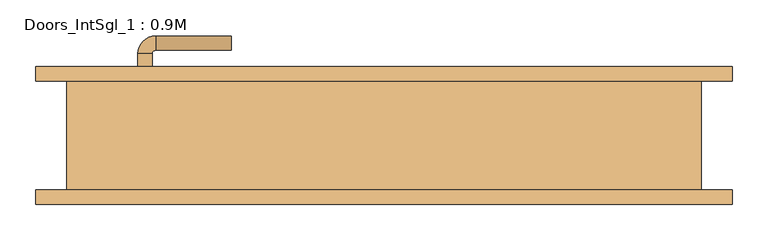
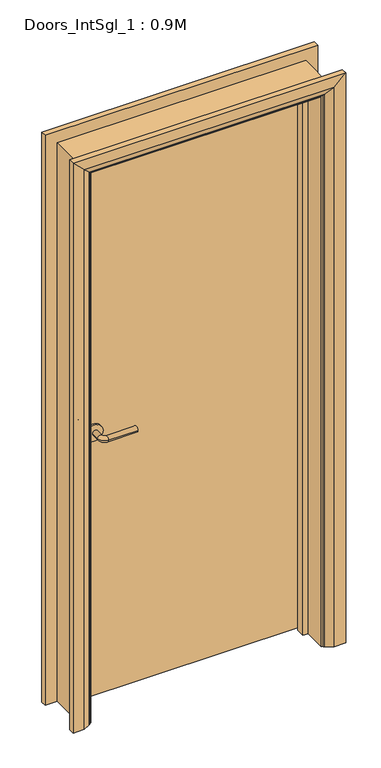
"""IFC4 building model written with IfcOpenShell, lengths in millimetres: door geometry, Doors_IntSgl_1 : 0.9M."""

from ifc_helpers import new_model, si_unit, point, frame, frame_2d, origin, place, context, project, spatial, polyline, circle_curve, ellipse_curve, trimmed, segment, composite_curve, outline, extrude, faceted_brep, source, transform, mapped, element, save
from ifc_brep_helpers import plane_surface, cylinder_surface, revolved_surface, advanced_brep


def doors_intsgl_1_0_9m_7aac3a70(model_context):
    return source(origin(), model_context, "Body", "SolidModel", [
        advanced_brep(
        [(-343.0, 30.2, 1000.0), (-323.0, 30.2, 1000.0), (-323.0, 0.2, 1000.0), (-343.0, 0.2, 1000.0), (-318.0, -4.8, 1000.0), (-318.0, -24.8, 1000.0), (-213.0, -24.8, 1000.0), (-213.0, -4.8, 1000.0)],
        [
            (0, 1, circle_curve(frame((-333.0, 30.2, 1000.0), z_axis=(0.0, 1.0, 0.0), x_axis=(1.0, 0.0, 0.0)), 10.0)),
            (1, 0, circle_curve(frame((-333.0, 30.2, 1000.0), z_axis=(0.0, 1.0, 0.0), x_axis=(1.0, 0.0, 0.0)), 10.0)),
            (1, 2),
            (2, 3, circle_curve(frame((-333.0, 0.2, 1000.0), z_axis=(0.0, 1.0, 0.0), x_axis=(1.0, 0.0, 0.0)), 10.0)),
            (3, 0),
            (3, 2, circle_curve(frame((-333.0, 0.2, 1000.0), z_axis=(0.0, 1.0, 0.0), x_axis=(1.0, 0.0, 0.0)), 10.0)),
            (4, 5, circle_curve(frame((-318.0, -14.8, 1000.0), z_axis=(-1.0, 0.0, 0.0), x_axis=(0.0, 1.0, 0.0)), 10.0)),
            (5, 3, circle_curve(frame((-318.0, 0.2, 1000.0), z_axis=(0.0, 0.0, -1.0), x_axis=(-1.0, 0.0, 0.0)), 25.0)),
            (2, 4, circle_curve(frame((-318.0, 0.2, 1000.0), z_axis=(0.0, 0.0, 1.0), x_axis=(-1.0, 0.0, 0.0)), 5.0)),
            (5, 4, circle_curve(frame((-318.0, -14.8, 1000.0), z_axis=(-1.0, 0.0, 0.0), x_axis=(0.0, 1.0, 0.0)), 10.0)),
            (6, 7, circle_curve(frame((-213.0, -14.8, 1000.0), z_axis=(1.0, 0.0, 0.0), x_axis=(0.0, 1.0, 0.0)), 10.0)),
            (7, 6, circle_curve(frame((-213.0, -14.8, 1000.0), z_axis=(1.0, 0.0, 0.0), x_axis=(0.0, 1.0, 0.0)), 10.0)),
            (4, 7),
            (6, 5),
        ],
        [
            plane_surface(frame((-333.0, 30.2, 1000.0), z_axis=(0.0, 1.0, 0.0), x_axis=(0.0, 0.0, 1.0))),
            cylinder_surface(frame((-333.0, 30.2, 1000.0), z_axis=(0.0, 1.0, 0.0), x_axis=(1.0, 0.0, 0.0)), 10.0),
            revolved_surface(trimmed(ellipse_curve(frame((-333.0, 0.2, 1000.0), z_axis=(0.0, -1.0, 0.0), x_axis=(1.0, 0.0, 0.0)), 10.0, 10.0), [point((-343.0, 0.2, 1000.0))], [point((-323.0, 0.2, 1000.0))], True, "CARTESIAN"), (-318.0, 0.2, 1000.0), (0.0, 0.0, -1.0)),
            revolved_surface(trimmed(ellipse_curve(frame((-333.0, 0.2, 1000.0), z_axis=(0.0, -1.0, 0.0), x_axis=(1.0, 0.0, 0.0)), 10.0, 10.0), [point((-323.0, 0.2, 1000.0))], [point((-343.0, 0.2, 1000.0))], True, "CARTESIAN"), (-318.0, 0.2, 1000.0), (0.0, 0.0, -1.0)),
            plane_surface(frame((-213.0, -14.8, 1000.0), z_axis=(1.0, 0.0, 0.0), x_axis=(0.0, 0.0, 1.0))),
            cylinder_surface(frame((-318.0, -14.8, 1000.0), z_axis=(-1.0, 0.0, 0.0), x_axis=(0.0, 1.0, 0.0)), 10.0),
        ],
        [
            (0, [[1, 2]]),
            (1, [[3, 4, 5, -2]]),
            (1, [[-5, 6, -3, -1]]),
            (2, [[7, 8, -4, 9]]),
            (3, [[10, -9, -6, -8]]),
            (4, [[11, 12]]),
            (5, [[13, -11, 14, -7]]),
            (5, [[-14, -12, -13, -10]]),
        ],
    ),
        extrude(outline(composite_curve([segment(trimmed(circle_curve(frame_2d((1000.0, -335.5)), 30.0), [point((1000.0, -365.5))], [point((1000.0, -305.5))], False, "CARTESIAN"), True, "CONTINUOUS"), segment(trimmed(circle_curve(frame_2d((1000.0, -335.5)), 30.0), [point((1000.0, -305.5))], [point((1000.0, -365.5))], False, "CARTESIAN"), True, "CONTINUOUS")], self_intersect=False)), frame((0.0, 30.2, 0.0), z_axis=(0.0, 1.0, 0.0), x_axis=(0.0, 0.0, 1.0)), (0.0, 0.0, 1.0), 8.0),
        advanced_brep(
        [(-343.0, 84.2, 1000.0), (-323.0, 84.2, 1000.0), (-343.0, 114.2, 1000.0), (-323.0, 114.2, 1000.0), (-318.0, 119.2, 1000.0), (-318.0, 139.2, 1000.0), (-213.0, 139.2, 1000.0), (-213.0, 119.2, 1000.0)],
        [
            (0, 1, circle_curve(frame((-333.0, 84.2, 1000.0), z_axis=(0.0, -1.0, 0.0), x_axis=(1.0, 0.0, 0.0)), 10.0)),
            (1, 0, circle_curve(frame((-333.0, 84.2, 1000.0), z_axis=(0.0, -1.0, 0.0), x_axis=(1.0, 0.0, 0.0)), 10.0)),
            (0, 2),
            (2, 3, circle_curve(frame((-333.0, 114.2, 1000.0), z_axis=(0.0, -1.0, 0.0), x_axis=(1.0, 0.0, 0.0)), 10.0)),
            (3, 1),
            (3, 2, circle_curve(frame((-333.0, 114.2, 1000.0), z_axis=(0.0, -1.0, 0.0), x_axis=(1.0, 0.0, 0.0)), 10.0)),
            (4, 3, circle_curve(frame((-318.0, 114.2, 1000.0), z_axis=(0.0, 0.0, 1.0), x_axis=(-1.0, 0.0, 0.0)), 5.0)),
            (2, 5, circle_curve(frame((-318.0, 114.2, 1000.0), z_axis=(0.0, 0.0, -1.0), x_axis=(-1.0, 0.0, 0.0)), 25.0)),
            (5, 4, circle_curve(frame((-318.0, 129.2, 1000.0), z_axis=(-1.0, 0.0, 0.0), x_axis=(0.0, -1.0, 0.0)), 10.0)),
            (4, 5, circle_curve(frame((-318.0, 129.2, 1000.0), z_axis=(-1.0, 0.0, 0.0), x_axis=(0.0, -1.0, 0.0)), 10.0)),
            (6, 7, circle_curve(frame((-213.0, 129.2, 1000.0), z_axis=(1.0, 0.0, 0.0), x_axis=(0.0, -1.0, 0.0)), 10.0)),
            (7, 6, circle_curve(frame((-213.0, 129.2, 1000.0), z_axis=(1.0, 0.0, 0.0), x_axis=(0.0, -1.0, 0.0)), 10.0)),
            (5, 6),
            (7, 4),
        ],
        [
            plane_surface(frame((-333.0, 84.2, 1000.0), z_axis=(0.0, -1.0, 0.0), x_axis=(0.0, 0.0, 1.0))),
            cylinder_surface(frame((-333.0, 84.2, 1000.0), z_axis=(0.0, -1.0, 0.0), x_axis=(1.0, 0.0, 0.0)), 10.0),
            revolved_surface(trimmed(ellipse_curve(frame((-333.0, 114.2, 1000.0), z_axis=(0.0, -1.0, 0.0), x_axis=(1.0, 0.0, 0.0)), 10.0, 10.0), [point((-343.0, 114.2, 1000.0))], [point((-323.0, 114.2, 1000.0))], True, "CARTESIAN"), (-318.0, 114.2, 1000.0), (0.0, 0.0, -1.0)),
            revolved_surface(trimmed(ellipse_curve(frame((-333.0, 114.2, 1000.0), z_axis=(0.0, -1.0, 0.0), x_axis=(1.0, 0.0, 0.0)), 10.0, 10.0), [point((-323.0, 114.2, 1000.0))], [point((-343.0, 114.2, 1000.0))], True, "CARTESIAN"), (-318.0, 114.2, 1000.0), (0.0, 0.0, -1.0)),
            plane_surface(frame((-213.0, 129.2, 1000.0), z_axis=(1.0, 0.0, 0.0), x_axis=(0.0, 0.0, 1.0))),
            cylinder_surface(frame((-318.0, 129.2, 1000.0), z_axis=(-1.0, 0.0, 0.0), x_axis=(0.0, -1.0, 0.0)), 10.0),
        ],
        [
            (0, [[1, 2]]),
            (1, [[-1, 3, 4, 5]]),
            (1, [[-2, -5, 6, -3]]),
            (2, [[7, -4, 8, 9]]),
            (3, [[-8, -6, -7, 10]]),
            (4, [[11, 12]]),
            (5, [[-9, 13, -12, 14]]),
            (5, [[-10, -14, -11, -13]]),
        ],
    ),
        extrude(outline(composite_curve([segment(trimmed(circle_curve(frame_2d((1000.0, -335.5)), 30.0), [point((1000.0, -365.5))], [point((1000.0, -305.5))], False, "CARTESIAN"), True, "CONTINUOUS"), segment(trimmed(circle_curve(frame_2d((1000.0, -335.5)), 30.0), [point((1000.0, -305.5))], [point((1000.0, -365.5))], False, "CARTESIAN"), True, "CONTINUOUS")], self_intersect=False)), frame((0.0, 76.2, 0.0), z_axis=(0.0, 1.0, 0.0), x_axis=(0.0, 0.0, 1.0)), (0.0, 0.0, 1.0), 8.0),
        extrude(outline(polyline([(408.0, 38.2), (-408.0, 38.2), (-408.0, 76.2), (408.0, 76.2), (408.0, 38.2)])), frame((0.0, 0.0, 8.0), z_axis=(0.0, 0.0, 1.0), x_axis=(1.0, 0.0, 0.0)), (0.0, 0.0, 1.0), 2060.0),
        faceted_brep([(-410.0, 76.2, 0.0), (-410.0, -76.2, 0.0), (-442.0, -76.2, 0.0), (-442.0, 76.2, 0.0), (-410.0, 76.2, 2070.0), (-410.0, -76.2, 2070.0), (-442.0, -76.2, 2102.0), (-442.0, 76.2, 2102.0), (410.0, 76.2, 0.0), (442.0, 76.2, 0.0), (442.0, -76.2, 0.0), (410.0, -76.2, 0.0), (410.0, 76.2, 2070.0), (442.0, 76.2, 2102.0), (442.0, -76.2, 2102.0), (410.0, -76.2, 2070.0)], [[[0, 1, 2, 3]], [[1, 0, 4, 5]], [[2, 1, 5, 6]], [[3, 2, 6, 7]], [[0, 3, 7, 4]], [[8, 9, 10, 11]], [[12, 13, 9, 8]], [[13, 14, 10, 9]], [[14, 15, 11, 10]], [[15, 12, 8, 11]], [[5, 4, 12, 15]], [[6, 5, 15, 14]], [[7, 6, 14, 13]], [[4, 7, 13, 12]]]),
        advanced_brep(
        [(-485.0, -96.2, 0.0), (-485.0, -76.2, 0.0), (-415.0, -76.2, 0.0), (-419.0, -82.2, 0.0), (-445.0, -96.2, 0.0), (-485.0, -96.2, 2145.0), (-485.0, -76.2, 2145.0), (-415.0, -76.2, 2075.0), (-419.0, -82.2, 2079.0), (-445.0, -96.2, 2105.0), (485.0, -96.2, 0.0), (445.0, -96.2, 0.0), (419.0, -82.2, 0.0), (415.0, -76.2, 0.0), (485.0, -76.2, 0.0), (485.0, -96.2, 2145.0), (445.0, -96.2, 2105.0), (419.0, -82.2, 2079.0), (415.0, -76.2, 2075.0), (485.0, -76.2, 2145.0)],
        [
            (0, 1),
            (1, 2),
            (2, 3, circle_curve(frame((-423.0, -75.2, 0.0), z_axis=(0.0, 0.0, -1.0), x_axis=(-1.0, 0.0, 0.0)), 8.0622577)),
            (3, 4),
            (4, 0),
            (0, 5),
            (5, 6),
            (6, 1),
            (6, 7),
            (7, 2),
            (7, 8, ellipse_curve(frame((-423.0, -75.2, 2083.0), z_axis=(-0.7071067811865475, 0.0, -0.7071067811865475), x_axis=(0.7071067811865474, 0.0, -0.7071067811865476)), 11.4017543, 8.0622577)),
            (8, 3),
            (8, 9),
            (9, 4),
            (9, 5),
            (10, 11),
            (11, 12),
            (12, 13, circle_curve(frame((423.0, -75.2, 0.0), z_axis=(0.0, 0.0, -1.0), x_axis=(1.0, 0.0, 0.0)), 8.0622577)),
            (13, 14),
            (14, 10),
            (15, 16),
            (16, 11),
            (10, 15),
            (16, 17),
            (17, 12),
            (17, 18, ellipse_curve(frame((423.0, -75.2, 2083.0), z_axis=(0.7071067811865475, 0.0, -0.7071067811865475), x_axis=(0.7071067811865474, 0.0, 0.7071067811865476)), 11.4017543, 8.0622577)),
            (18, 13),
            (18, 19),
            (19, 14),
            (19, 15),
            (5, 15),
            (19, 6),
            (18, 7),
            (17, 8),
            (16, 9),
        ],
        [
            plane_surface(frame((-415.0, -149.0010989, 0.0), z_axis=(0.0, 0.0, -1.0), x_axis=(1.0, 0.0, 0.0))),
            plane_surface(frame((-485.0, -96.2, 0.0), z_axis=(-1.0, 0.0, 0.0), x_axis=(0.0, 0.0, 1.0))),
            plane_surface(frame((-485.0, -76.2, 0.0), z_axis=(0.0, 1.0, 0.0), x_axis=(0.0, 0.0, 1.0))),
            cylinder_surface(frame((-423.0, -75.2, 0.0), z_axis=(0.0, 0.0, -1.0), x_axis=(-1.0, 0.0, 0.0)), 8.0622577),
            plane_surface(frame((-419.0, -82.2, 0.0), z_axis=(0.4740998230350183, -0.8804710999221749, 0.0), x_axis=(0.0, 0.0, 1.0))),
            plane_surface(frame((-445.0, -96.2, 0.0), z_axis=(0.0, -1.0, 0.0), x_axis=(0.0, 0.0, 1.0))),
            plane_surface(frame((415.0, -149.0010989, 0.0), z_axis=(0.0, 0.0, -1.0), x_axis=(-1.0, 0.0, 0.0))),
            plane_surface(frame((445.0, -96.2, 2105.0), z_axis=(0.0, -1.0, 0.0), x_axis=(0.0, 0.0, -1.0))),
            plane_surface(frame((419.0, -82.2, 2079.0), z_axis=(-0.4740998230350183, -0.8804710999221749, 0.0), x_axis=(0.0, 0.0, -1.0))),
            cylinder_surface(frame((423.0, -75.2, 2075.0), z_axis=(0.0, 0.0, 1.0), x_axis=(1.0, 0.0, 0.0)), 8.0622577),
            plane_surface(frame((485.0, -76.2, 2145.0), z_axis=(0.0, 1.0, 0.0), x_axis=(0.0, 0.0, -1.0))),
            plane_surface(frame((485.0, -96.2, 2145.0), z_axis=(1.0, 0.0, 0.0), x_axis=(0.0, 0.0, -1.0))),
            plane_surface(frame((-485.0, -96.2, 2145.0), z_axis=(0.0, 0.0, 1.0), x_axis=(1.0, 0.0, 0.0))),
            plane_surface(frame((-485.0, -76.2, 2145.0), z_axis=(0.0, 1.0, 0.0), x_axis=(1.0, 0.0, 0.0))),
            cylinder_surface(frame((-415.0, -75.2, 2083.0), z_axis=(-1.0, 0.0, 0.0), x_axis=(0.0, 0.0, 1.0)), 8.0622577),
            plane_surface(frame((-419.0, -82.2, 2079.0), z_axis=(0.0, -0.8804710999221749, -0.4740998230350183), x_axis=(1.0, 0.0, 0.0))),
            plane_surface(frame((-445.0, -96.2, 2105.0), z_axis=(0.0, -1.0, 0.0), x_axis=(1.0, 0.0, 0.0))),
        ],
        [
            (0, [[1, 2, 3, 4, 5]]),
            (1, [[-1, 6, 7, 8]]),
            (2, [[-2, -8, 9, 10]]),
            (3, [[-3, -10, 11, 12]]),
            (4, [[-4, -12, 13, 14]]),
            (5, [[-5, -14, 15, -6]]),
            (6, [[16, 17, 18, 19, 20]]),
            (7, [[21, 22, -16, 23]]),
            (8, [[24, 25, -17, -22]]),
            (9, [[26, 27, -18, -25]]),
            (10, [[28, 29, -19, -27]]),
            (11, [[30, -23, -20, -29]]),
            (12, [[-7, 31, -30, 32]]),
            (13, [[-9, -32, -28, 33]]),
            (14, [[-11, -33, -26, 34]]),
            (15, [[-13, -34, -24, 35]]),
            (16, [[-15, -35, -21, -31]]),
        ],
    ),
        extrude(outline(polyline([(0.0, -410.0), (0.0, -391.0), (2051.0, -391.0), (2051.0, 391.0), (0.0, 391.0), (0.0, 410.0), (2070.0, 410.0), (2070.0, -410.0), (0.0, -410.0)])), frame((0.0, 4.2, 0.0), z_axis=(0.0, 1.0, 0.0), x_axis=(0.0, 0.0, 1.0)), (0.0, 0.0, 1.0), 32.0),
        advanced_brep(
        [(485.0, 96.2, 0.0), (485.0, 76.2, 0.0), (415.0, 76.2, 0.0), (419.0, 82.2, 0.0), (445.0, 96.2, 0.0), (485.0, 96.2, 2145.0), (485.0, 76.2, 2145.0), (-485.0, 76.2, 2145.0), (-485.0, 76.2, 0.0), (-415.0, 76.2, 0.0), (-415.0, 76.2, 2075.0), (415.0, 76.2, 2075.0), (419.0, 82.2, 2079.0), (445.0, 96.2, 2105.0), (-445.0, 96.2, 2105.0), (-445.0, 96.2, 0.0), (-485.0, 96.2, 0.0), (-485.0, 96.2, 2145.0), (-419.0, 82.2, 0.0), (-419.0, 82.2, 2079.0)],
        [
            (0, 1),
            (1, 2),
            (2, 3, circle_curve(frame((423.0, 75.2, 0.0), z_axis=(0.0, 0.0, -1.0), x_axis=(1.0, 0.0, 0.0)), 8.0622577)),
            (3, 4),
            (4, 0),
            (0, 5),
            (5, 6),
            (6, 1),
            (6, 7),
            (7, 8),
            (8, 9),
            (9, 10),
            (10, 11),
            (11, 2),
            (11, 12, ellipse_curve(frame((423.0, 75.2, 2083.0), z_axis=(0.7071067811865475, 0.0, -0.7071067811865475), x_axis=(-0.7071067811865474, 0.0, -0.7071067811865476)), 11.4017543, 8.0622577)),
            (12, 3),
            (12, 13),
            (13, 4),
            (13, 14),
            (14, 15),
            (15, 16),
            (16, 17),
            (17, 5),
            (7, 17),
            (16, 8),
            (15, 18),
            (18, 9, circle_curve(frame((-423.0, 75.2, 0.0), z_axis=(0.0, 0.0, -1.0), x_axis=(-1.0, 0.0, 0.0)), 8.0622577)),
            (19, 10, ellipse_curve(frame((-423.0, 75.2, 2083.0), z_axis=(-0.7071067811865475, 0.0, -0.7071067811865475), x_axis=(-0.7071067811865474, 0.0, 0.7071067811865476)), 11.4017543, 8.0622577)),
            (18, 19),
            (14, 19),
            (19, 12),
        ],
        [
            plane_surface(frame((415.0, 76.2, 0.0), z_axis=(0.0, 0.0, -1.0), x_axis=(0.0, -1.0, 0.0))),
            plane_surface(frame((485.0, 96.2, 0.0), z_axis=(1.0, 0.0, 0.0), x_axis=(0.0, 0.0, 1.0))),
            plane_surface(frame((485.0, 76.2, 0.0), z_axis=(0.0, -1.0, 0.0), x_axis=(0.0, 0.0, 1.0))),
            cylinder_surface(frame((423.0, 75.2, 0.0), z_axis=(0.0, 0.0, -1.0), x_axis=(1.0, 0.0, 0.0)), 8.0622577),
            plane_surface(frame((419.0, 82.2, 0.0), z_axis=(-0.4740998230350126, 0.880471099922178, 0.0), x_axis=(0.0, 0.0, 1.0))),
            plane_surface(frame((445.0, 96.2, 0.0), z_axis=(0.0, 1.0, 0.0), x_axis=(0.0, 0.0, 1.0))),
            plane_surface(frame((-485.0, 96.2, 2145.0), z_axis=(-1.0, 0.0, 0.0), x_axis=(0.0, 0.0, -1.0))),
            plane_surface(frame((-415.0, 76.2, 0.0), z_axis=(0.0, 0.0, -1.0), x_axis=(0.0, -1.0, 0.0))),
            cylinder_surface(frame((-423.0, 75.2, 2075.0), z_axis=(0.0, 0.0, 1.0), x_axis=(-1.0, 0.0, 0.0)), 8.0622577),
            plane_surface(frame((-419.0, 82.2, 2079.0), z_axis=(0.47409982303501824, 0.8804710999221749, 0.0), x_axis=(0.0, 0.0, -1.0))),
            plane_surface(frame((485.0, 96.2, 2145.0), z_axis=(0.0, 0.0, 1.0), x_axis=(-1.0, 0.0, 0.0))),
            cylinder_surface(frame((415.0, 75.2, 2083.0), z_axis=(1.0, 0.0, 0.0), x_axis=(0.0, 0.0, 1.0)), 8.0622577),
            plane_surface(frame((419.0, 82.2, 2079.0), z_axis=(0.0, 0.8804710999221764, -0.4740998230350154), x_axis=(-1.0, 0.0, 0.0))),
        ],
        [
            (0, [[1, 2, 3, 4, 5]]),
            (1, [[-1, 6, 7, 8]]),
            (2, [[-2, -8, 9, 10, 11, 12, 13, 14]]),
            (3, [[-3, -14, 15, 16]]),
            (4, [[-4, -16, 17, 18]]),
            (5, [[-5, -18, 19, 20, 21, 22, 23, -6]]),
            (6, [[24, -22, 25, -10]]),
            (7, [[-21, 26, 27, -11, -25]]),
            (8, [[28, -12, -27, 29]]),
            (9, [[30, -29, -26, -20]]),
            (10, [[-7, -23, -24, -9]]),
            (11, [[-15, -13, -28, 31]]),
            (12, [[-17, -31, -30, -19]]),
        ],
    ),
    ])


if __name__ == "__main__":
    model = new_model("IFC4")
    model_context = context("Model", 3, world=origin())
    ifc_project = project(units=[si_unit("LENGTHUNIT", "METRE", prefix="MILLI")], contexts=[model_context])
    site = spatial("IfcSite", under=ifc_project)
    building = spatial("IfcBuilding", under=site)
    placement = place(None, origin())
    doors_intsgl_1_0_9m_shape = doors_intsgl_1_0_9m_7aac3a70(model_context)
    element("IfcDoor", 1, ObjectType="Doors_IntSgl_1 : 0.9M", at=placement, inside=building, context=model_context, shape_type="MappedRepresentation", body=[
        mapped(doors_intsgl_1_0_9m_shape, transform((0.0, 0.0, 0.0), x_axis=(1.0, 0.0, 0.0), y_axis=(0.0, 1.0, 0.0), z_axis=(0.0, 0.0, 1.0))),
    ])
    save(model, "model.ifc")

# Revit data of these elements
# Type "Doors_IntSgl_1 : 0.9M"
#   Type Mark = "57"
#   Type Comments = "Internal Single"
#   Operation = "SingleSwingRight"
#   Construction Type Id = "MDOOR"
#   Manufacturer = "Revit"
#   Keynote = "L20"
#   Description = "Internal Single Door"
#   Analytic Construction = "Metal"
#   UnderCut = 0.008 m
#   Tolerance = 0.002 m
#   Thickness = 0.038 m
#   Structural Tolerance = 0.008 m
#   StopDepth = 0.032 m
#   Stop Thickness = 0.019 m
#   Rough Width = 0.9 m
#   Rough Height = 2.11 m
#   Height to Top Lock Rail = 1.0 m
#   Heat Transfer Coefficient (U) = 3.7021 W/(m²·K)
#   Handle Z Distance = 1.0 m
#   Handle X Distance = 0.075 m
#   Frame Thickness = 0.032 m
#   Door Panel Width = 0.816 m
#   Door Panel Thickness = 0.038 m
#   Door Panel Offset = 0.0 m
#   Height = 2.11 m
#   Width = 0.9 m
#   Door Panel Height = 2.06 m
#   Architrave Setback = 0.005 m
#   Vis - Ironmongery = yes
#   Define Thermal Properties by = 1
#   Material Ironmongery = Door - Handle
#   Material Frame = Door - Frame/Mullion
#   Material Door = Door - Panel
#   Material Architrave = Door - Architrave
#   Visual Light Transmittance = 0
#   Solar Heat Gain Coefficient = 0
#   Function = (empty or 0)
#   Wall Closure = (empty or 0)
# Element 1 (IfcDoor, "Doors_IntSgl_1 : 0.9M")
#   Materials on its faces: "Door - Architrave", "Door - Handle", "Door - Frame/Mullion", "Door - Panel"
# Materials
#   "Door - Handle": colour RGB 0 0 0, transparency 0, Keynote = "P21", Cost = 0
#   "Door - Frame/Mullion": class "Wood", colour RGB 212 179 113, transparency 0, Keynote = "L20", Cost = 0
#   "Door - Panel": class "Wood", colour RGB 210 159 95, transparency 0, Keynote = "L20", Cost = 0
#   "Door - Architrave": class "Wood", colour RGB 154 90 5, transparency 0, Keynote = "P20", Cost = 0
